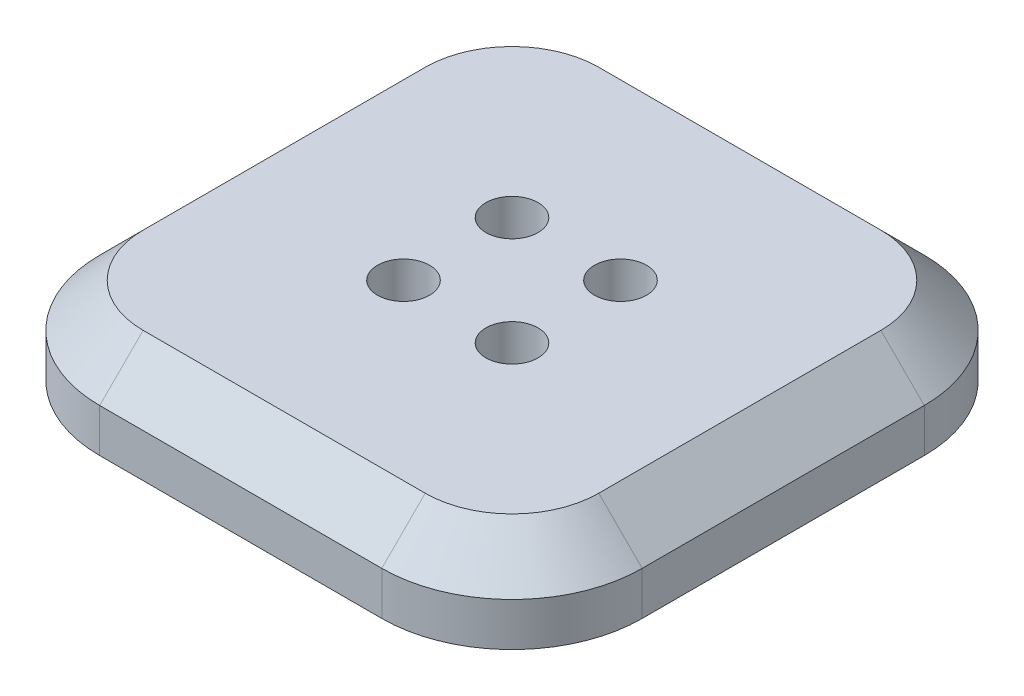
from build123d import *

# Parameters (mm, degrees)
BASE_PLATE_PROFILE_125X125_W = 125
BASE_PLATE_PROFILE_125X125_H = 125
BASE_PLATE_20MM_DEPTH        = 20
CORNER_FILLETS_R30_R         = 30
EDGE_CHAMFER_10X45_SIZE      = 10
DOWEL_HOLES_12X10_A_D        = 12
DOWEL_HOLES_12X10_A_DEPTH    = 10
DOWEL_HOLES_12X10_A_TIP      = 3.605163714
DOWEL_HOLES_12X10_B_D        = 12
DOWEL_HOLES_12X10_B_DEPTH    = 10
DOWEL_HOLES_12X10_B_TIP      = 3.605163714


with BuildPart() as part:
    # Base Plate Profile 125x125 → Base Plate 20mm (new body)
    with BuildSketch(Plane(origin=(0, 0, 0), x_dir=(1, 0, 0), z_dir=(0, 1, 0))):
        Rectangle(BASE_PLATE_PROFILE_125X125_W, BASE_PLATE_PROFILE_125X125_H)
    extrude(amount=BASE_PLATE_20MM_DEPTH)

    # Corner Fillets R30
    corner_fillets_r30_edges = [part.edges().sort_by_distance(p)[0] for p in [
        (62.5, 10, 62.5),
        (-62.5, 10, 62.5),
        (-62.5, 10, -62.5),
        (62.5, 10, -62.5),
    ]]
    fillet(corner_fillets_r30_edges, radius=CORNER_FILLETS_R30_R)

    # Edge Chamfer 10x45°
    edge_chamfer_10x45_edges = [part.edges().sort_by_distance(p)[0] for p in [
        (-62.5, 20, 0),
        (0, 20, -62.5),
        (62.5, 20, 0),
        (0, 20, 62.5),
        (-53.713203436, 20, 53.713203436),
        (53.713203436, 20, 53.713203436),
        (53.713203436, 20, -53.713203436),
        (-53.713203436, 20, -53.713203436),
    ]]
    chamfer(edge_chamfer_10x45_edges, length=EDGE_CHAMFER_10X45_SIZE)

    # Dowel Holes Ø12x10 A
    with Locations(Plane(origin=(-12.5, 20, -12.5), x_dir=(0, 0, 1), z_dir=(0, 1, 0))):
        with Locations((0, 0), (0, 25), (25, 25), (25, 0)):
            Hole(DOWEL_HOLES_12X10_A_D / 2, depth=DOWEL_HOLES_12X10_A_DEPTH)
            with Locations((0, 0, -(DOWEL_HOLES_12X10_A_DEPTH + DOWEL_HOLES_12X10_A_TIP / 2))):  # 118° drill point
                Cone(0, DOWEL_HOLES_12X10_A_D / 2, DOWEL_HOLES_12X10_A_TIP, mode=Mode.SUBTRACT)

    # Dowel Holes Ø12x10 B
    with Locations(Plane(origin=(-37.5, 0, 37.5), x_dir=(0, 0, -1), z_dir=(0, -1, 0))):
        with Locations((0, 0), (0, 75), (75, 75), (75, 0)):
            Hole(DOWEL_HOLES_12X10_B_D / 2, depth=DOWEL_HOLES_12X10_B_DEPTH)
            with Locations((0, 0, -(DOWEL_HOLES_12X10_B_DEPTH + DOWEL_HOLES_12X10_B_TIP / 2))):  # 118° drill point
                Cone(0, DOWEL_HOLES_12X10_B_D / 2, DOWEL_HOLES_12X10_B_TIP, mode=Mode.SUBTRACT)


solid = part.part
